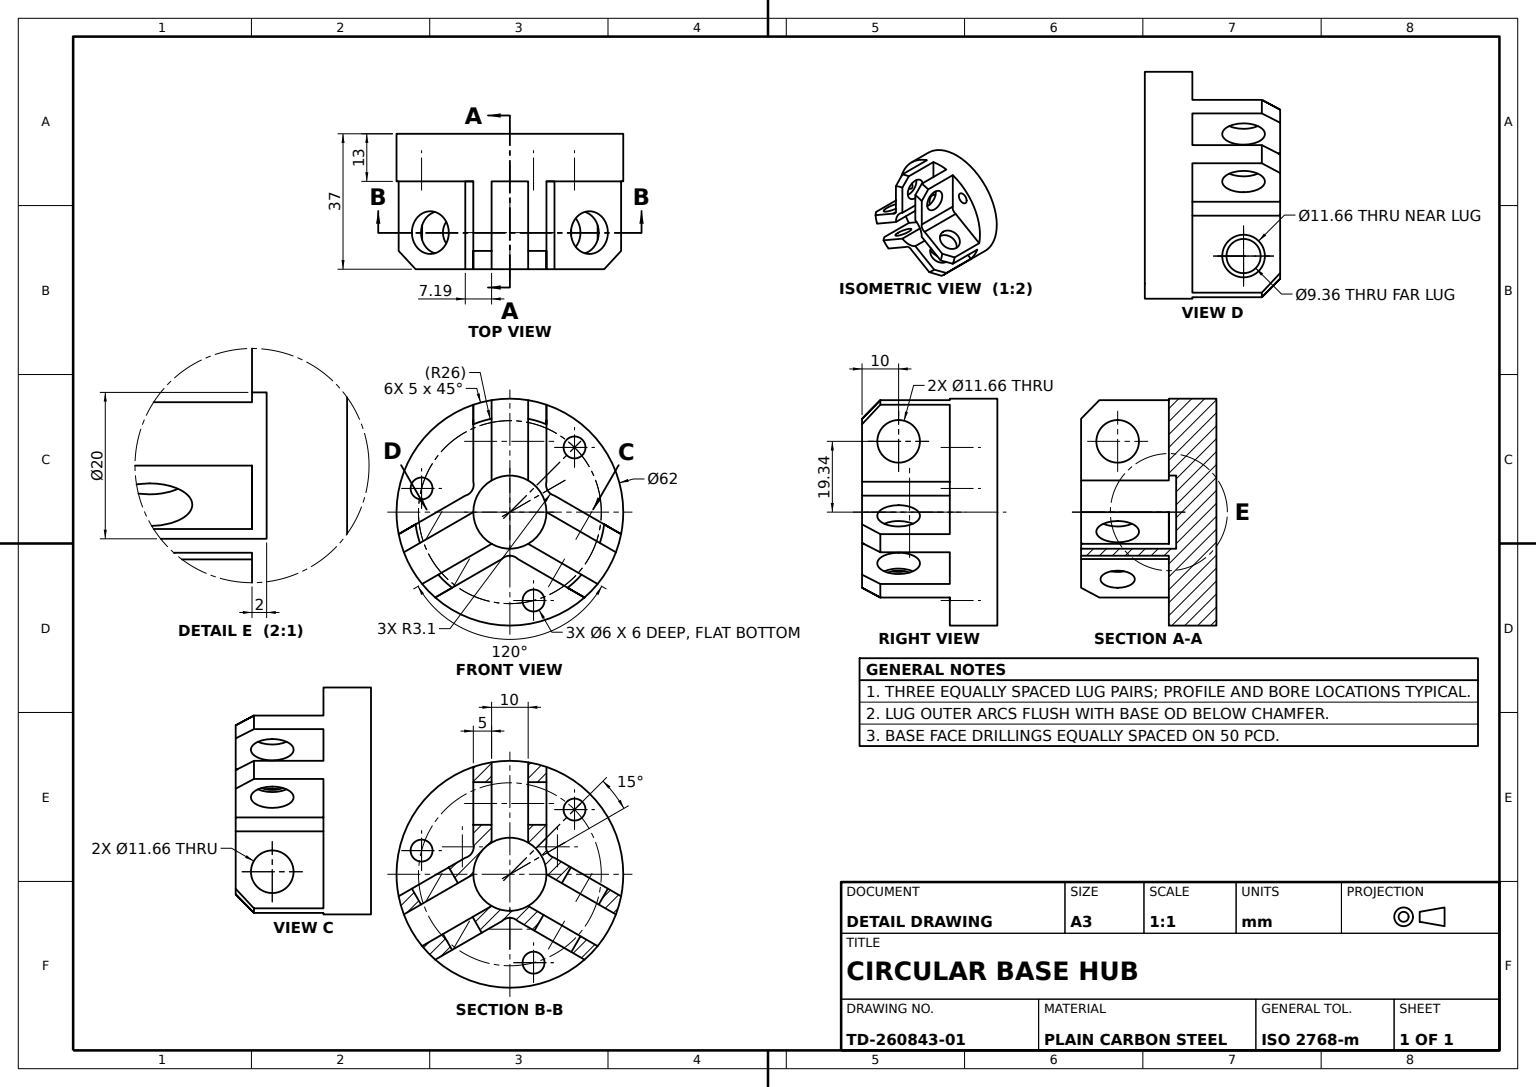
from build123d import *
from build123d.topology import SkipClean

# Parameters (mm, degrees)
BASE_DISC_SKETCH_R         = 31
BASE_DISC_DEPTH            = 13
BASE_SLOT_SKETCH_3X_R      = 3
BASE_SLOTS_3X_DEPTH        = 6
CLAMP_START                = -24
CLAMP_LUG_DEPTH            = 24
LUG_HOLE_A_SKETCH_R        = 4.680098696
LUG_HOLE_A_DEPTH           = 57.727418415
LUG_HOLE_B_SKETCH_R        = 5.830404683
LUG_HOLE_B_DEPTH           = 59.693575035
CLAMP_LUG_PATTERN_3X_COUNT = 3
FACE_RECESS_SKETCH_R       = 10
FACE_RECESS_2MM_DEPTH      = 2
LUG_CHAMFER_5MM_SIZE       = 5


with BuildPart() as part:
    # Base Disc Sketch → Base Disc (new body)
    with BuildSketch(Plane.XY):
        with Locations(Location((0, 0, 0), (0, 0, 180))):
            Circle(BASE_DISC_SKETCH_R)
    extrude(amount=BASE_DISC_DEPTH)

    # Base Slot Sketch 3x → Base Slots 3x (cut)
    with BuildSketch(Plane.XY):
        with Locations((-6.470476128, -24.148145657)):
            Circle(BASE_SLOT_SKETCH_3X_R)
        with Locations((-17.67766953, 17.67766953)):
            Circle(BASE_SLOT_SKETCH_3X_R)
        with Locations((24.148145657, 6.470476128)):
            Circle(BASE_SLOT_SKETCH_3X_R)
    extrude(amount=BASE_SLOTS_3X_DEPTH, mode=Mode.SUBTRACT)

    # Clamp Lug Sketch → Clamp Lug (add)
    with SkipClean():  # the faces are left unmerged after this step: merging them gives an invalid solid
        with BuildSketch(Plane.XY.offset(CLAMP_START)):
            with BuildLine():
                Line((5, 8.660254038), (5, 30.594117082))
                ThreePointArc((5, 30.594117082), (7.526051267, 30.072554802), (10, 29.342801502))
                Line((10, 29.342801502), (10, 8.306623863))
                ThreePointArc((10, 8.306623863), (10.309933784, 5.952443046), (12.193747285, 4.506942106))
                Line((12.193747285, 4.506942106), (30.411611519, -6.011146713))
                ThreePointArc((30.411611519, -6.011146713), (29.806622049, -8.518525814), (28.995282599, -10.966931522))
                Line((28.995282599, -10.966931522), (10, 0))
                ThreePointArc((10, 0), (8.660254038, 5), (5, 8.660254038))
            make_face()
        clamp_lug = extrude(amount=CLAMP_LUG_DEPTH)

    # Lug Hole A Sketch → Lug Hole A (cut, through all)
    with SkipClean():  # the faces are left unmerged after this step: merging them gives an invalid solid
        with BuildSketch(Plane(origin=(10, 0, 0), x_dir=(0, 0, -1), z_dir=(1, 0, 0))):
            with Locations(Location((14, 19.342801502, 0), (0, 0, 90))):
                Circle(LUG_HOLE_A_SKETCH_R)
        lug_hole_a = extrude(amount=-LUG_HOLE_A_DEPTH, mode=Mode.SUBTRACT)

    # Lug Hole B Sketch → Lug Hole B (cut, through all)
    with SkipClean():  # the faces are left unmerged after this step: merging them gives an invalid solid
        with BuildSketch(Plane(origin=(5, 8.660254038, 0), x_dir=(0.8660254037844388, -0.4999999999999998, 0), z_dir=(0.4999999999999998, 0.8660254037844388, 0))):
            with Locations(Location((19.342801502, 14, 0), (0, 0, 180))):
                Circle(LUG_HOLE_B_SKETCH_R)
        lug_hole_b = extrude(amount=-LUG_HOLE_B_DEPTH, mode=Mode.SUBTRACT)

    # Clamp Lug Pattern 3x: Clamp Lug, Lug Hole A, Lug Hole B ×3 about axis
    with SkipClean():  # the faces are left unmerged after this step: merging them gives an invalid solid
        clamp_lug_pattern_3x_axis = Axis((0, 0, 0), (0, 0, 1))
        add([clamp_lug.rotate(clamp_lug_pattern_3x_axis, i * 360 / CLAMP_LUG_PATTERN_3X_COUNT) for i in range(1, CLAMP_LUG_PATTERN_3X_COUNT)])
        add([lug_hole_a.rotate(clamp_lug_pattern_3x_axis, i * 360 / CLAMP_LUG_PATTERN_3X_COUNT) for i in range(1, CLAMP_LUG_PATTERN_3X_COUNT)], mode=Mode.SUBTRACT)
        add([lug_hole_b.rotate(clamp_lug_pattern_3x_axis, i * 360 / CLAMP_LUG_PATTERN_3X_COUNT) for i in range(1, CLAMP_LUG_PATTERN_3X_COUNT)], mode=Mode.SUBTRACT)

    # Face Recess Sketch → Face Recess 2mm (cut)
    with SkipClean():  # the faces are left unmerged after this step: merging them gives an invalid solid
        with BuildSketch(Plane(origin=(0, 0, 0), x_dir=(-1, 0, 0), z_dir=(0, 0, -1))):
            Circle(FACE_RECESS_SKETCH_R)
        extrude(amount=-FACE_RECESS_2MM_DEPTH, mode=Mode.SUBTRACT)

    # Lug Chamfer 5mm
    lug_chamfer_5mm_edges = [part.edges().sort_by_distance(p)[0] for p in [
        (7.526051267, 30.072554802, -24),
        (29.806622049, -8.518525814, -24),
        (-29.806622049, -8.518525814, -24),
        (-7.526051267, 30.072554802, -24),
        (22.280570782, -21.554028988, -24),
        (-22.280570782, -21.554028988, -24),
    ]]
    chamfer(lug_chamfer_5mm_edges, length=LUG_CHAMFER_5MM_SIZE)


solid = part.part
